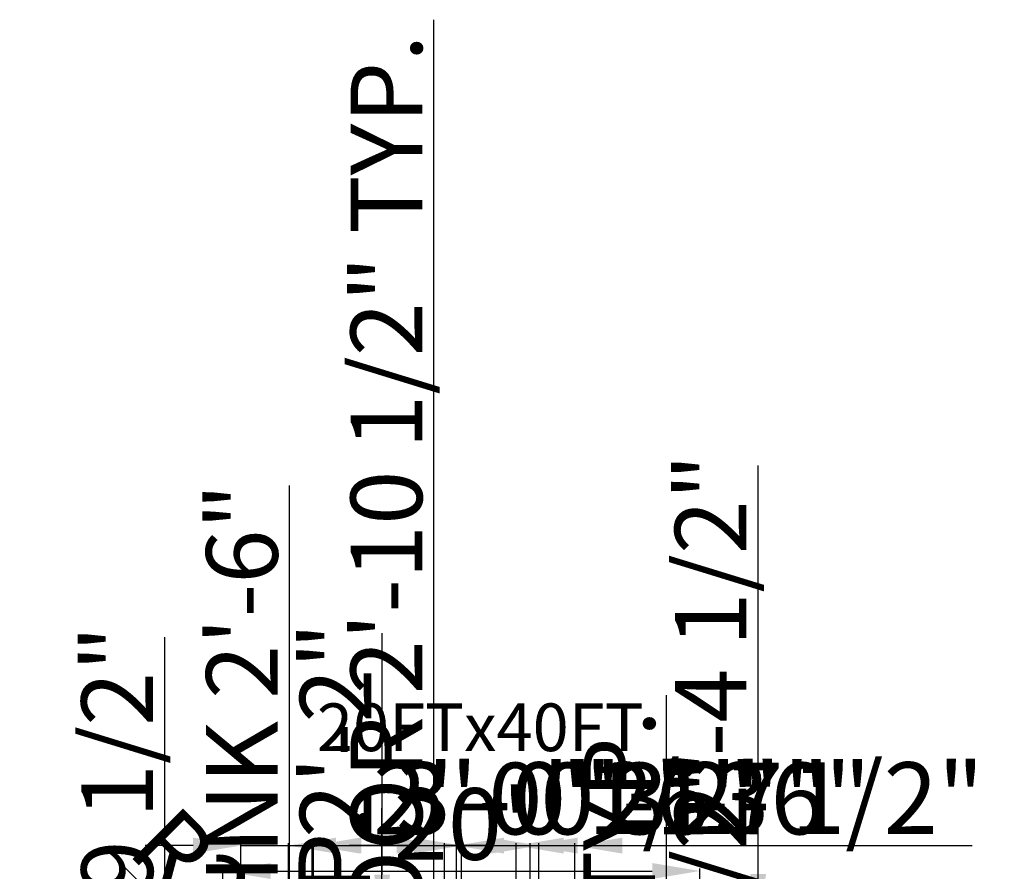
# Model space of a CAD drawing. Units: inches. Extents: x 1102 to 2414, y 295 to 1561.
# Tile 10 of 11: x 1475 to 1971, y 1133 to 1561. Entities that reach past the tile are written whole.
import ezdxf

# ---------------------------------------------------------------- set-up
doc = ezdxf.new("R2010")
doc.units = ezdxf.units.IN
doc.layers.add('A-ANNO-DIMS', color=2, linetype='Continuous', lineweight=18)
doc.layers.add('A-ANNO-TEXT', color=7, linetype='Continuous', lineweight=35)
doc.styles.get("Standard").update_dxf_attribs({"font": 'arial.ttf'})
doc.dimstyles.new('ISO-25', dxfattribs={"dimtxt": 36, "dimasz": 24, "dimexe": 1.25, "dimexo": 0.625, "dimtad": 1, "dimlunit": 4, "dimtxsty": 'Standard', "dimcen": 2.5, "dimadec": 0, "dimazin": 0, "dimtfac": 1, "dimtmove": 0, "dimatfit": 3, "dimfxl": 1, "dimarcsym": 0})

# ---------------------------------------------------------------- blocks, each defined once
blk = doc.blocks.new('*D1')
at = {"layer": 'A-ANNO-DIMS', "color": 0, "lineweight": -2, "transparency": 16777216}
for p, q in [((1577.54, 1117.38), (1577.54, 1134.48)), ((1817.54, 1117.38), (1817.54, 1134.48)), ((1601.54, 1133.23), (1793.54, 1133.23))]:
    blk.add_line(p, q, dxfattribs=at)
at = {"layer": 'A-ANNO-DIMS', "color": 0, "transparency": 16777216}
for points in [[(1601.54, 1137.23), (1601.54, 1129.23), (1577.54, 1133.23)], [(1793.54, 1137.23), (1793.54, 1129.23), (1817.54, 1133.23)]]:
    blk.add_solid(points, dxfattribs=at)
at = {"layer": 'Defpoints', "color": 0, "transparency": 16777216}
for p in [(1817.54, 1133.23), (1577.54, 1116.76), (1817.54, 1116.76)]:
    blk.add_point(p, dxfattribs=at)
at = {"layer": 'A-ANNO-DIMS', "color": 0, "transparency": 16777216, "insert": (1697.54, 1152.24), "char_height": 36, "attachment_point": 5}
blk.add_mtext("20'", dxfattribs=at)
blk = doc.blocks.new('*D25')
at = {"layer": 'A-ANNO-DIMS', "color": 0, "lineweight": -2, "transparency": 16777216}
for p, q in [((1800.76, 877.69), (1800.76, 1221.61)), ((1796.43, 853.69), (1802.01, 853.69)), ((1800.76, 820.65), (1800.76, 853.69)), ((1796.43, 820.65), (1802.01, 820.65)), ((1800.76, 796.65), (1800.76, 772.65))]:
    blk.add_line(p, q, dxfattribs=at)
at = {"layer": 'A-ANNO-DIMS', "color": 0, "transparency": 16777216}
for points in [[(1796.76, 877.69), (1804.76, 877.69), (1800.76, 853.69)], [(1796.76, 796.65), (1804.76, 796.65), (1800.76, 820.65)]]:
    blk.add_solid(points, dxfattribs=at)
at = {"layer": 'Defpoints', "color": 0, "transparency": 16777216}
for p in [(1795.81, 853.69), (1800.76, 853.69), (1795.81, 820.65)]:
    blk.add_point(p, dxfattribs=at)
at = {"layer": 'A-ANNO-DIMS', "color": 0, "transparency": 16777216, "insert": (1781.53, 1061.65), "char_height": 36, "attachment_point": 5, "rotation": 90}
blk.add_mtext('WC 2\'-9" TYP.', dxfattribs=at)
blk = doc.blocks.new('*D27')
at = {"layer": 'A-ANNO-DIMS', "color": 0, "lineweight": -2, "transparency": 16777216}
for p, q in [((1683.72, 1041.76), (1683.72, 1561.36)), ((1679.17, 1017.76), (1684.97, 1017.76)), ((1683.72, 983.26), (1683.72, 1017.76)), ((1679.17, 983.26), (1684.97, 983.26)), ((1683.72, 959.26), (1683.72, 935.26))]:
    blk.add_line(p, q, dxfattribs=at)
at = {"layer": 'A-ANNO-DIMS', "color": 0, "transparency": 16777216}
for points in [[(1679.72, 1041.76), (1687.72, 1041.76), (1683.72, 1017.76)], [(1679.72, 959.26), (1687.72, 959.26), (1683.72, 983.26)]]:
    blk.add_solid(points, dxfattribs=at)
at = {"layer": 'Defpoints', "color": 0, "transparency": 16777216}
for p in [(1678.54, 1017.76), (1683.72, 1017.76), (1678.54, 983.26)]:
    blk.add_point(p, dxfattribs=at)
at = {"layer": 'A-ANNO-DIMS', "color": 0, "transparency": 16777216, "insert": (1664.47, 1313.56), "char_height": 36, "attachment_point": 5, "rotation": 90}
blk.add_mtext('DOOR 2\'-10 1/2" TYP.', dxfattribs=at)
blk = doc.blocks.new('*D32')
at = {"layer": 'A-ANNO-DIMS', "color": 0, "lineweight": -2, "transparency": 16777216}
for p, q in [((1657.46, 811.76), (1657.46, 1164.91)), ((1654.49, 787.76), (1658.71, 787.76)), ((1657.46, 765.26), (1657.46, 787.76)), ((1654.49, 765.26), (1658.71, 765.26)), ((1657.46, 741.26), (1657.46, 717.26))]:
    blk.add_line(p, q, dxfattribs=at)
at = {"layer": 'A-ANNO-DIMS', "color": 0, "transparency": 16777216}
for points in [[(1653.46, 811.76), (1661.46, 811.76), (1657.46, 787.76)], [(1653.46, 741.26), (1661.46, 741.26), (1657.46, 765.26)]]:
    blk.add_solid(points, dxfattribs=at)
at = {"layer": 'Defpoints', "color": 0, "transparency": 16777216}
for p in [(1653.86, 787.76), (1657.46, 787.76), (1653.86, 765.26)]:
    blk.add_point(p, dxfattribs=at)
at = {"layer": 'A-ANNO-DIMS', "color": 0, "transparency": 16777216, "insert": (1638.22, 1000.34), "char_height": 36, "attachment_point": 5, "rotation": 90}
blk.add_mtext('1\'-10 1/2" TYP.', dxfattribs=at)
blk = doc.blocks.new('*D33')
at = {"layer": 'A-ANNO-DIMS', "color": 0, "lineweight": -2, "transparency": 16777216}
for p, q in [((1623.16, 1080.7), (1623.16, 1075.57)), ((1653.16, 1080.7), (1653.16, 1075.57)), ((1599.16, 1076.82), (1575.16, 1076.82)), ((1623.16, 1076.82), (1653.16, 1076.82)), ((1677.16, 1076.82), (1989.06, 1076.82))]:
    blk.add_line(p, q, dxfattribs=at)
at = {"layer": 'A-ANNO-DIMS', "color": 0, "transparency": 16777216}
for points in [[(1599.16, 1080.82), (1599.16, 1072.82), (1623.16, 1076.82)], [(1677.16, 1080.82), (1677.16, 1072.82), (1653.16, 1076.82)]]:
    blk.add_solid(points, dxfattribs=at)
at = {"layer": 'Defpoints', "color": 0, "transparency": 16777216}
for p in [(1623.16, 1081.32), (1653.16, 1081.32), (1653.16, 1076.82)]:
    blk.add_point(p, dxfattribs=at)
at = {"layer": 'A-ANNO-DIMS', "color": 0, "transparency": 16777216, "insert": (1845.11, 1096.06), "char_height": 36, "attachment_point": 5}
blk.add_mtext('RANGE 2\'-6"', dxfattribs=at)
blk = doc.blocks.new('*D34')
at = {"layer": 'A-ANNO-DIMS', "color": 0, "lineweight": -2, "transparency": 16777216}
for p, q in [((1657.66, 1131.32), (1657.66, 1252.88)), ((1653.79, 1107.32), (1658.91, 1107.32)), ((1657.66, 1081.32), (1657.66, 1107.32)), ((1653.79, 1081.32), (1658.91, 1081.32)), ((1657.66, 1057.32), (1657.66, 1033.32))]:
    blk.add_line(p, q, dxfattribs=at)
at = {"layer": 'A-ANNO-DIMS', "color": 0, "transparency": 16777216}
for points in [[(1653.66, 1131.32), (1661.66, 1131.32), (1657.66, 1107.32)], [(1653.66, 1057.32), (1661.66, 1057.32), (1657.66, 1081.32)]]:
    blk.add_solid(points, dxfattribs=at)
at = {"layer": 'Defpoints', "color": 0, "transparency": 16777216}
for p in [(1653.16, 1107.32), (1657.66, 1107.32), (1653.16, 1081.32)]:
    blk.add_point(p, dxfattribs=at)
at = {"layer": 'A-ANNO-DIMS', "color": 0, "transparency": 16777216, "insert": (1638.96, 1204.1), "char_height": 36, "attachment_point": 5, "rotation": 90}
blk.add_mtext('2\'-2"', dxfattribs=at)
blk = doc.blocks.new('*D35')
at = {"layer": 'A-ANNO-DIMS', "color": 0, "lineweight": -2, "transparency": 16777216}
for p, q in [((1611.04, 1074.99), (1611.04, 1327.12)), ((1607.17, 1050.99), (1612.29, 1050.99)), ((1611.04, 1020.99), (1611.04, 1050.99)), ((1607.17, 1020.99), (1612.29, 1020.99)), ((1611.04, 996.99), (1611.04, 972.99))]:
    blk.add_line(p, q, dxfattribs=at)
at = {"layer": 'A-ANNO-DIMS', "color": 0, "transparency": 16777216}
for points in [[(1607.04, 1074.99), (1615.04, 1074.99), (1611.04, 1050.99)], [(1607.04, 996.99), (1615.04, 996.99), (1611.04, 1020.99)]]:
    blk.add_solid(points, dxfattribs=at)
at = {"layer": 'Defpoints', "color": 0, "transparency": 16777216}
for p in [(1606.54, 1050.99), (1611.04, 1050.99), (1606.54, 1020.99)]:
    blk.add_point(p, dxfattribs=at)
at = {"layer": 'A-ANNO-DIMS', "color": 0, "transparency": 16777216, "insert": (1591.81, 1213.06), "char_height": 36, "attachment_point": 5, "rotation": 90}
blk.add_mtext('SINK 2\'-6"', dxfattribs=at)
blk = doc.blocks.new('*D45')
at = {"layer": 'A-ANNO-DIMS', "color": 0, "lineweight": -2, "transparency": 16777216}
for p, q in [((1712.54, 1146.01), (1688.54, 1146.01)), ((1736.54, 770.38), (1736.54, 1147.26)), ((1736.54, 1146.01), (1754.54, 1146.01)), ((1754.54, 770.38), (1754.54, 1147.26)), ((1778.54, 1146.01), (1896.1, 1146.01))]:
    blk.add_line(p, q, dxfattribs=at)
at = {"layer": 'A-ANNO-DIMS', "color": 0, "transparency": 16777216}
for points in [[(1712.54, 1150.01), (1712.54, 1142.01), (1736.54, 1146.01)], [(1778.54, 1150.01), (1778.54, 1142.01), (1754.54, 1146.01)]]:
    blk.add_solid(points, dxfattribs=at)
at = {"layer": 'Defpoints', "color": 0, "transparency": 16777216}
for p in [(1754.54, 1146.01), (1736.54, 769.76), (1754.54, 769.76)]:
    blk.add_point(p, dxfattribs=at)
at = {"layer": 'A-ANNO-DIMS', "color": 0, "transparency": 16777216, "insert": (1849.32, 1165.02), "char_height": 36, "attachment_point": 5}
blk.add_mtext('1\'-6"', dxfattribs=at)
blk = doc.blocks.new('*D48')
at = {"layer": 'A-ANNO-DIMS', "color": 0, "lineweight": -2, "transparency": 16777216}
for p, q in [((1665.04, 1146.01), (1641.04, 1146.01)), ((1689.04, 854.38), (1689.04, 1147.26)), ((1689.04, 1146.01), (1732.04, 1146.01)), ((1732.04, 858.88), (1732.04, 1147.26)), ((1756.04, 1146.01), (1876.97, 1146.01))]:
    blk.add_line(p, q, dxfattribs=at)
at = {"layer": 'A-ANNO-DIMS', "color": 0, "transparency": 16777216}
for points in [[(1665.04, 1150.01), (1665.04, 1142.01), (1689.04, 1146.01)], [(1756.04, 1150.01), (1756.04, 1142.01), (1732.04, 1146.01)]]:
    blk.add_solid(points, dxfattribs=at)
at = {"layer": 'Defpoints', "color": 0, "transparency": 16777216}
for p in [(1732.04, 1146.01), (1732.04, 858.26), (1689.04, 853.76)]:
    blk.add_point(p, dxfattribs=at)
at = {"layer": 'A-ANNO-DIMS', "color": 0, "transparency": 16777216, "insert": (1828.51, 1165.03), "char_height": 36, "attachment_point": 5}
blk.add_mtext('3\'-7"', dxfattribs=at)
blk = doc.blocks.new('*D49')
at = {"layer": 'A-ANNO-DIMS', "color": 0, "lineweight": -2, "transparency": 16777216}
for p, q in [((1846.79, 983.26), (1846.79, 1188.29)), ((1809.17, 983.26), (1848.04, 983.26)), ((1846.79, 934.76), (1846.79, 959.26)), ((1809.17, 910.76), (1848.04, 910.76))]:
    blk.add_line(p, q, dxfattribs=at)
at = {"layer": 'A-ANNO-DIMS', "color": 0, "transparency": 16777216}
for points in [[(1842.79, 959.26), (1850.79, 959.26), (1846.79, 983.26)], [(1842.79, 934.76), (1850.79, 934.76), (1846.79, 910.76)]]:
    blk.add_solid(points, dxfattribs=at)
at = {"layer": 'Defpoints', "color": 0, "transparency": 16777216}
for p in [(1808.54, 983.26), (1846.79, 983.26), (1808.54, 910.76)]:
    blk.add_point(p, dxfattribs=at)
at = {"layer": 'A-ANNO-DIMS', "color": 0, "transparency": 16777216, "insert": (1827.56, 1097.77), "char_height": 36, "attachment_point": 5, "rotation": 90}
blk.add_mtext('6\'-0 1/2"', dxfattribs=at)
blk = doc.blocks.new('*D51')
at = {"layer": 'A-ANNO-DIMS', "color": 0, "lineweight": -2, "transparency": 16777216}
for p, q in [((1665.04, 1146.01), (1641.04, 1146.01)), ((1689.04, 988.38), (1689.04, 1147.26)), ((1689.04, 1146.01), (1695.04, 1146.01)), ((1695.04, 988.38), (1695.04, 1147.26)), ((1719.04, 1146.01), (1839.99, 1146.01))]:
    blk.add_line(p, q, dxfattribs=at)
at = {"layer": 'A-ANNO-DIMS', "color": 0, "transparency": 16777216}
for points in [[(1665.04, 1150.01), (1665.04, 1142.01), (1689.04, 1146.01)], [(1719.04, 1150.01), (1719.04, 1142.01), (1695.04, 1146.01)]]:
    blk.add_solid(points, dxfattribs=at)
at = {"layer": 'Defpoints', "color": 0, "transparency": 16777216}
for p in [(1695.04, 1146.01), (1689.04, 987.76), (1695.04, 987.76)]:
    blk.add_point(p, dxfattribs=at)
at = {"layer": 'A-ANNO-DIMS', "color": 0, "transparency": 16777216, "insert": (1791.52, 1165.02), "char_height": 36, "attachment_point": 5}
blk.add_mtext('0\'-6"', dxfattribs=at)
blk = doc.blocks.new('*D53')
at = {"layer": 'A-ANNO-DIMS', "color": 0, "lineweight": -2, "transparency": 16777216}
for p, q in [((1562.54, 1146.01), (1538.54, 1146.01)), ((1586.54, 988.38), (1586.54, 1147.26)), ((1586.54, 1146.01), (1610.54, 1146.01)), ((1610.54, 988.38), (1610.54, 1147.26)), ((1634.54, 1146.01), (1756.11, 1146.01))]:
    blk.add_line(p, q, dxfattribs=at)
at = {"layer": 'A-ANNO-DIMS', "color": 0, "transparency": 16777216}
for points in [[(1562.54, 1150.01), (1562.54, 1142.01), (1586.54, 1146.01)], [(1634.54, 1150.01), (1634.54, 1142.01), (1610.54, 1146.01)]]:
    blk.add_solid(points, dxfattribs=at)
at = {"layer": 'Defpoints', "color": 0, "transparency": 16777216}
for p in [(1610.54, 1146.01), (1586.54, 987.76), (1610.54, 987.76)]:
    blk.add_point(p, dxfattribs=at)
at = {"layer": 'A-ANNO-DIMS', "color": 0, "transparency": 16777216, "insert": (1707.32, 1165.02), "char_height": 36, "attachment_point": 5}
blk.add_mtext('2\'-0"', dxfattribs=at)
blk = doc.blocks.new('*D54')
at = {"layer": 'A-ANNO-DIMS', "color": 0, "lineweight": -2, "transparency": 16777216}
for p, q in [((1846.79, 1131.76), (1846.79, 1337.21)), ((1685.17, 1107.76), (1848.04, 1107.76)), ((1846.79, 1079.39), (1846.79, 1107.76)), ((1685.17, 1079.39), (1848.04, 1079.39)), ((1846.79, 1055.39), (1846.79, 1031.39))]:
    blk.add_line(p, q, dxfattribs=at)
at = {"layer": 'A-ANNO-DIMS', "color": 0, "transparency": 16777216}
for points in [[(1842.79, 1131.76), (1850.79, 1131.76), (1846.79, 1107.76)], [(1842.79, 1055.39), (1850.79, 1055.39), (1846.79, 1079.39)]]:
    blk.add_solid(points, dxfattribs=at)
at = {"layer": 'Defpoints', "color": 0, "transparency": 16777216}
for p in [(1684.54, 1107.76), (1846.79, 1107.76), (1684.54, 1079.39)]:
    blk.add_point(p, dxfattribs=at)
at = {"layer": 'A-ANNO-DIMS', "color": 0, "transparency": 16777216, "insert": (1827.56, 1246.48), "char_height": 36, "attachment_point": 5, "rotation": 90}
blk.add_mtext('2\'-4 1/2"', dxfattribs=at)
blk = doc.blocks.new('*D55')
at = {"layer": 'A-ANNO-DIMS', "color": 0, "lineweight": -2, "transparency": 16777216}
for p, q in [((1562.54, 1146.01), (1538.54, 1146.01)), ((1586.54, 722.38), (1586.54, 1147.26)), ((1586.54, 1146.01), (1622.54, 1146.01)), ((1622.54, 722.38), (1622.54, 1147.26)), ((1646.54, 1146.01), (1767.47, 1146.01))]:
    blk.add_line(p, q, dxfattribs=at)
at = {"layer": 'A-ANNO-DIMS', "color": 0, "transparency": 16777216}
for points in [[(1562.54, 1150.01), (1562.54, 1142.01), (1586.54, 1146.01)], [(1646.54, 1150.01), (1646.54, 1142.01), (1622.54, 1146.01)]]:
    blk.add_solid(points, dxfattribs=at)
at = {"layer": 'Defpoints', "color": 0, "transparency": 16777216}
for p in [(1622.54, 1146.01), (1586.54, 721.76), (1622.54, 721.76)]:
    blk.add_point(p, dxfattribs=at)
at = {"layer": 'A-ANNO-DIMS', "color": 0, "transparency": 16777216, "insert": (1719.01, 1165.03), "char_height": 36, "attachment_point": 5}
blk.add_mtext('3\'-0"', dxfattribs=at)
blk = doc.blocks.new('*D60')
at = {"layer": 'A-ANNO-DIMS', "color": 0, "lineweight": -2, "transparency": 16777216}
for p, q in [((1562.54, 1146.01), (1538.54, 1146.01)), ((1586.54, 1108.38), (1586.54, 1147.26)), ((1586.54, 1146.01), (1623.16, 1146.01)), ((1623.16, 1107.95), (1623.16, 1147.26)), ((1647.16, 1146.01), (1851.97, 1146.01))]:
    blk.add_line(p, q, dxfattribs=at)
at = {"layer": 'A-ANNO-DIMS', "color": 0, "transparency": 16777216}
for points in [[(1562.54, 1150.01), (1562.54, 1142.01), (1586.54, 1146.01)], [(1647.16, 1150.01), (1647.16, 1142.01), (1623.16, 1146.01)]]:
    blk.add_solid(points, dxfattribs=at)
at = {"layer": 'Defpoints', "color": 0, "transparency": 16777216}
for p in [(1623.16, 1146.01), (1586.54, 1107.76), (1623.16, 1107.32)]:
    blk.add_point(p, dxfattribs=at)
at = {"layer": 'A-ANNO-DIMS', "color": 0, "transparency": 16777216, "insert": (1761.57, 1165.26), "char_height": 36, "attachment_point": 5}
blk.add_mtext('3\'-0 1/2"', dxfattribs=at)
blk = doc.blocks.new('*D61')
at = {"layer": 'A-ANNO-DIMS', "color": 0, "lineweight": -2, "transparency": 16777216}
for p, q in [((1548.29, 1045.43), (1548.29, 1250.88)), ((1586.36, 1021.43), (1547.04, 1021.43)), ((1548.29, 987.76), (1548.29, 1021.43)), ((1585.92, 987.76), (1547.04, 987.76)), ((1548.29, 963.76), (1548.29, 939.76))]:
    blk.add_line(p, q, dxfattribs=at)
at = {"layer": 'A-ANNO-DIMS', "color": 0, "transparency": 16777216}
for points in [[(1544.29, 1045.43), (1552.29, 1045.43), (1548.29, 1021.43)], [(1544.29, 963.76), (1552.29, 963.76), (1548.29, 987.76)]]:
    blk.add_solid(points, dxfattribs=at)
at = {"layer": 'Defpoints', "color": 0, "transparency": 16777216}
for p in [(1548.29, 1021.43), (1586.98, 1021.43), (1586.54, 987.76)]:
    blk.add_point(p, dxfattribs=at)
at = {"layer": 'A-ANNO-DIMS', "color": 0, "transparency": 16777216, "insert": (1529.06, 1160.15), "char_height": 36, "attachment_point": 5, "rotation": 90}
blk.add_mtext('2\'-9 1/2"', dxfattribs=at)
blk = doc.blocks.new('*D65')
at = {"layer": 'A-ANNO-DIMS', "color": 0, "lineweight": -2, "transparency": 16777216}
for p, q in [((1673.64, 1146.01), (1649.64, 1146.01)), ((1697.64, 770.38), (1697.64, 1147.26)), ((1697.64, 1146.01), (1725.04, 1146.01)), ((1725.04, 770.38), (1725.04, 1147.26)), ((1749.04, 1146.01), (1954.49, 1146.01))]:
    blk.add_line(p, q, dxfattribs=at)
at = {"layer": 'A-ANNO-DIMS', "color": 0, "transparency": 16777216}
for points in [[(1673.64, 1150.01), (1673.64, 1142.01), (1697.64, 1146.01)], [(1749.04, 1150.01), (1749.04, 1142.01), (1725.04, 1146.01)]]:
    blk.add_solid(points, dxfattribs=at)
at = {"layer": 'Defpoints', "color": 0, "transparency": 16777216}
for p in [(1725.04, 1146.01), (1697.64, 769.76), (1725.04, 769.76)]:
    blk.add_point(p, dxfattribs=at)
at = {"layer": 'A-ANNO-DIMS', "color": 0, "transparency": 16777216, "insert": (1863.77, 1165.26), "char_height": 36, "attachment_point": 5}
blk.add_mtext('2\'-3 1/2"', dxfattribs=at)
blk = doc.blocks.new('*D68')
at = {"layer": 'A-ANNO-DIMS', "color": 0, "lineweight": -2, "transparency": 16777216}
for p, q in [((1527.48, 1135.83), (1637.36, 1025.94)), ((1675.54, 987.76), (1654.33, 1008.97))]:
    blk.add_line(p, q, dxfattribs=at)
at = {"layer": 'A-ANNO-DIMS', "color": 0, "transparency": 16777216}
blk.add_solid([(1640.19, 1028.77), (1634.53, 1023.12), (1654.33, 1008.97)], dxfattribs=at)
at = {"layer": 'Defpoints', "color": 0, "transparency": 16777216}
for p in [(1654.33, 1008.97), (1675.54, 987.76)]:
    blk.add_point(p, dxfattribs=at)
at = {"layer": 'A-ANNO-DIMS', "color": 0, "transparency": 16777216, "insert": (1587.37, 1102.81), "char_height": 36, "attachment_point": 5, "rotation": 314.9996}
blk.add_mtext('R2\'-6"', dxfattribs=at)

msp = doc.modelspace()

# ---------------------------------------------------------------- texts
at = {"layer": 'A-ANNO-TEXT', "insert": (1624.849, 1217.505), "char_height": 24, "attachment_point": 1}
msp.add_mtext_dynamic_manual_height_columns('20FTx40FT', width=50.64919, gutter_width=12.5, heights=[0], dxfattribs=at)

# ---------------------------------------------------------------- dimensions: what is measured, and where the dimension line sits
at = {"layer": 'A-ANNO-DIMS'}
for base, p1, p2, text, picture, middle in [((1683.719, 1017.76), (1678.544, 983.26), (1678.544, 1017.76), 'DOOR <> TYP.', '*D27', (1664.468, 1313.559)), ((1611.044, 1050.991), (1606.544, 1020.991), (1606.544, 1050.991), 'SINK <>', '*D35', (1591.805, 1213.055)), ((1800.764, 853.692), (1795.807, 820.646), (1795.807, 853.692), 'WC <> TYP.', '*D25', (1781.525, 1061.653)), ((1657.464, 787.76), (1653.864, 765.26), (1653.864, 787.76), '<> TYP.', '*D32', (1638.225, 1000.337))]:
    dim = msp.add_linear_dim(base=base, p1=p1, p2=p2, angle=90, text=text, dimstyle='ISO-25', override={"dimdec": 1, "dimlfac": 1, "dimrnd": 0, "dimzin": 1, "dimdsep": 46, "dimlunit": 4, "dimfrac": 2}, dxfattribs=at)
    dim.commit()
    dim.dimension.update_dxf_attribs({"geometry": picture, "text_midpoint": middle})
for base, p1, p2, picture, middle in [((1846.794, 1107.76), (1684.544, 1079.395), (1684.544, 1107.76), '*D54', (1827.555, 1246.483)), ((1657.662, 1107.321), (1653.162, 1081.321), (1653.162, 1107.321), '*D34', (1638.964, 1204.102)), ((1548.294, 1021.43), (1586.544, 987.76), (1586.983, 1021.43), '*D61', (1529.055, 1160.153)), ((1846.794, 983.26), (1808.544, 910.76), (1808.544, 983.26), '*D49', (1827.555, 1097.774))]:
    dim = msp.add_linear_dim(base=base, p1=p1, p2=p2, angle=90, dimstyle='ISO-25', override={"dimdec": 1, "dimlfac": 1, "dimrnd": 0, "dimzin": 1, "dimdsep": 46, "dimlunit": 4, "dimfrac": 2}, dxfattribs=at)
    dim.commit()
    dim.dimension.update_dxf_attribs({"geometry": picture, "text_midpoint": middle})
for base, p1, p2, override, picture, middle in [((1623.162, 1146.01), (1586.544, 1107.76), (1623.162, 1107.321), {"dimdec": 1, "dimlfac": 1, "dimrnd": 0, "dimzin": 1, "dimdsep": 46, "dimlunit": 4, "dimfrac": 2}, '*D60', (1761.566, 1165.261)), ((1725.044, 1146.01), (1697.644, 769.76), (1725.044, 769.76), {"dimdec": 1, "dimlfac": 1, "dimrnd": 0, "dimzin": 1, "dimdsep": 46, "dimlunit": 4, "dimfrac": 2}, '*D65', (1863.767, 1165.261)), ((1622.544, 1146.01), (1586.544, 721.76), (1622.544, 721.76), {"dimdec": 1, "dimlfac": 1, "dimrnd": 0, "dimzin": 1, "dimdsep": 46, "dimlunit": 4, "dimfrac": 2}, '*D55', (1719.005, 1165.028)), ((1610.544, 1146.01), (1586.544, 987.76), (1610.544, 987.76), {"dimdec": 1, "dimlfac": 1, "dimrnd": 0, "dimzin": 1, "dimdsep": 46, "dimlunit": 4, "dimfrac": 2}, '*D53', (1707.325, 1165.015)), ((1732.044, 1146.01), (1689.044, 853.76), (1732.044, 858.26), {"dimdec": 1, "dimlfac": 1, "dimrnd": 0, "dimzin": 1, "dimdsep": 46, "dimlunit": 4, "dimfrac": 2}, '*D48', (1828.505, 1165.028)), ((1695.044, 1146.01), (1689.044, 987.76), (1695.044, 987.76), {"dimdec": 1, "dimlfac": 1, "dimrnd": 0, "dimzin": 1, "dimdsep": 46, "dimlunit": 4, "dimfrac": 2}, '*D51', (1791.518, 1165.015)), ((1754.544, 1146.01), (1736.544, 769.76), (1754.544, 769.76), {"dimdec": 1, "dimlfac": 1, "dimrnd": 0, "dimzin": 1, "dimdsep": 46, "dimlunit": 4, "dimfrac": 2}, '*D45', (1849.323, 1165.015)), ((1817.544, 1133.235), (1577.544, 1116.76), (1817.544, 1116.76), {"dimclrd": 0, "dimclre": 0, "dimclrt": 0}, '*D1', (1697.544, 1152.24))]:
    dim = msp.add_linear_dim(base=base, p1=p1, p2=p2, dimstyle='ISO-25', override=override, dxfattribs=at)
    dim.commit()
    dim.dimension.update_dxf_attribs({"geometry": picture, "text_midpoint": middle})
dim = msp.add_radius_dim(center=(1675.544, 987.76), mpoint=(1654.331, 1008.973), dimstyle='ISO-25', override={"dimdec": 1, "dimlfac": 1, "dimrnd": 0, "dimzin": 1, "dimdsep": 46, "dimlunit": 4, "dimfrac": 2}, dxfattribs=at)
dim.commit()
dim.dimension.update_dxf_attribs({"geometry": '*D68', "text_midpoint": (1587.373, 1102.811)})
dim = msp.add_linear_dim(base=(1653.162, 1076.821), p1=(1623.162, 1081.321), p2=(1653.162, 1081.321), text='RANGE <>', dimstyle='ISO-25', override={"dimdec": 1, "dimlfac": 1, "dimrnd": 0, "dimzin": 1, "dimdsep": 46, "dimlunit": 4, "dimfrac": 2}, dxfattribs=at)
dim.commit()
dim.dimension.update_dxf_attribs({"geometry": '*D33', "text_midpoint": (1845.112, 1096.06)})

doc.saveas('drawing.dxf')
